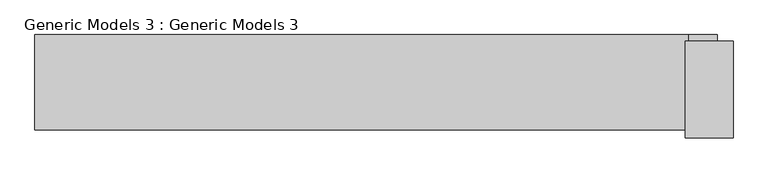
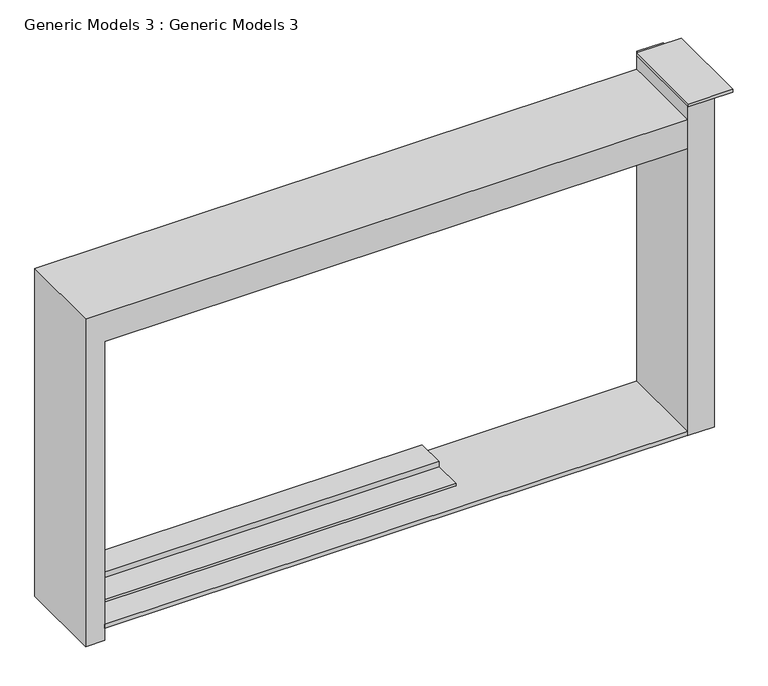
"""IFC4 building model written with IfcOpenShell, lengths in millimetres: proxy geometry, Generic Models 3 : Generic Models 3."""

from ifc_helpers import new_model, si_unit, frame, origin, place, context, project, spatial, polyline, outline, extrude, faceted_brep, source, transform, mapped, element, save


def generic_models_3_generic_models_3_3f7da236(model_context):
    return source(origin(), model_context, "Body", "SolidModel", [
        extrude(outline(polyline([(-4059.0995706, -12626.5777232), (-4059.0995706, -11851.8777232), (-3675.4859258, -11851.8777232), (-3675.4859258, -12626.5777232), (-4059.0995706, -12626.5777232)])), frame((0.0, 0.0, 3214.2510456), z_axis=(0.0, 0.0, 1.0), x_axis=(1.0, 0.0, 0.0)), (0.0, 0.0, 1.0), 25.4),
        faceted_brep([(-9263.4859258, -12563.0777232, 36.0466226), (-9098.3859258, -12563.0777232, 36.0466226), (-9098.3859258, -12563.0777232, 2781.5010692), (-4031.0859258, -12563.0777232, 2781.5010692), (-4031.0859258, -12563.0777232, 3048.0), (-9263.4859258, -12563.0777232, 3048.0), (-3802.4859258, -11801.0777232, 146.3632195), (-4031.0859258, -11801.0777232, 146.3632195), (-4031.0859258, -11801.0777232, 2781.5010692), (-9098.3859258, -11801.0777232, 2781.5010692), (-9098.3859258, -11801.0777232, 36.0466226), (-9263.4859258, -11801.0777232, 36.0466226), (-9263.4859258, -11801.0777232, 3048.0), (-4031.0859258, -11801.0777232, 3048.0), (-4031.0859258, -11801.0777232, 3214.2510456), (-3802.4859258, -11801.0777232, 3214.2510456), (-3802.4859258, -12568.2052445, 3214.2510456), (-3802.4859258, -12568.2052445, 146.3632195), (-4031.0859258, -12568.2052445, 3214.2510456), (-4031.0859258, -12568.2052445, 146.3632195)], [[[0, 1, 2, 3, 4, 5]], [[6, 7, 8, 9, 10, 11, 12, 13, 14, 15]], [[6, 15, 16, 17]], [[12, 5, 4, 13]], [[5, 12, 11, 0]], [[2, 9, 8, 3]], [[11, 10, 1, 0]], [[1, 10, 9, 2]], [[18, 16, 15, 14]], [[19, 7, 6, 17]], [[16, 18, 19, 17]], [[18, 14, 13, 4, 3, 8, 7, 19]]]),
        faceted_brep([(-5897.9859258, -11801.0777232, 146.3632195), (-5897.9859258, -12309.0777232, 146.3632195), (-5897.9859258, -12309.0777232, 182.2891808), (-5897.9859258, -11801.0777232, 182.2891808), (-5643.9859258, -11801.0777232, 146.3632195), (-5643.9859258, -12309.0777232, 146.3632195), (-4031.0859258, -12309.0777232, 146.3632195), (-4031.0859258, -12563.0777232, 146.3632195), (-9098.3859258, -12563.0777232, 146.3632195), (-9098.3859258, -12309.0777232, 146.3632195), (-9098.3859258, -12309.0777232, 182.2891808), (-9098.3859258, -12563.0777232, 182.2891808), (-4031.0859258, -12563.0777232, 182.2891808), (-4031.0859258, -11801.0777232, 182.2891808), (-4031.0859258, -11801.0777232, 144.1891808), (-5643.9859258, -11801.0777232, 144.1891808), (-4031.0859258, -12309.0777232, 144.1891808), (-5643.9859258, -12309.0777232, 144.1891808)], [[[0, 1, 2, 3]], [[1, 0, 4, 5, 6, 7, 8, 9]], [[3, 2, 10, 11, 12, 13]], [[0, 3, 13, 14, 15, 4]], [[8, 7, 12, 11]], [[9, 10, 2, 1]], [[13, 12, 7, 6, 16, 14]], [[8, 11, 10, 9]], [[15, 17, 5, 4]], [[17, 16, 6, 5]], [[14, 16, 17, 15]]]),
        extrude(outline(polyline([(-5897.9859258, -12309.0777232), (-9098.3859258, -12309.0777232), (-9098.3859258, -12055.0777232), (-5897.9859258, -12055.0777232), (-5897.9859258, -12309.0777232)])), frame((0.0, 0.0, 152.4), z_axis=(0.0, 0.0, 1.0), x_axis=(1.0, 0.0, 0.0)), (0.0, 0.0, 1.0), 49.681554),
        extrude(outline(polyline([(-5897.9859258, -12055.0777232), (-9098.3859258, -12055.0777232), (-9098.3859258, -11801.0777232), (-5897.9859258, -11801.0777232), (-5897.9859258, -12055.0777232)])), frame((0.0, 0.0, 152.4), z_axis=(0.0, 0.0, 1.0), x_axis=(1.0, 0.0, 0.0)), (0.0, 0.0, 1.0), 98.1871084),
    ])


if __name__ == "__main__":
    model = new_model("IFC4")
    model_context = context("Model", 3, world=origin())
    ifc_project = project(units=[si_unit("LENGTHUNIT", "METRE", prefix="MILLI")], contexts=[model_context])
    site = spatial("IfcSite", under=ifc_project)
    building = spatial("IfcBuilding", under=site)
    placement = place(None, origin())
    generic_models_3_generic_models_3_shape = generic_models_3_generic_models_3_3f7da236(model_context)
    element("IfcBuildingElementProxy", 1, Name="Generic Models 3 : Generic Models 3", ObjectType="Generic Models 3 : Generic Models 3", at=placement, inside=building, context=model_context, shape_type="MappedRepresentation", body=[
        mapped(generic_models_3_generic_models_3_shape, transform((0.0, 0.0, 0.0), x_axis=(1.0, 0.0, 0.0), y_axis=(0.0, 1.0, 0.0), z_axis=(0.0, 0.0, 1.0))),
    ])
    save(model, "model.ifc")
